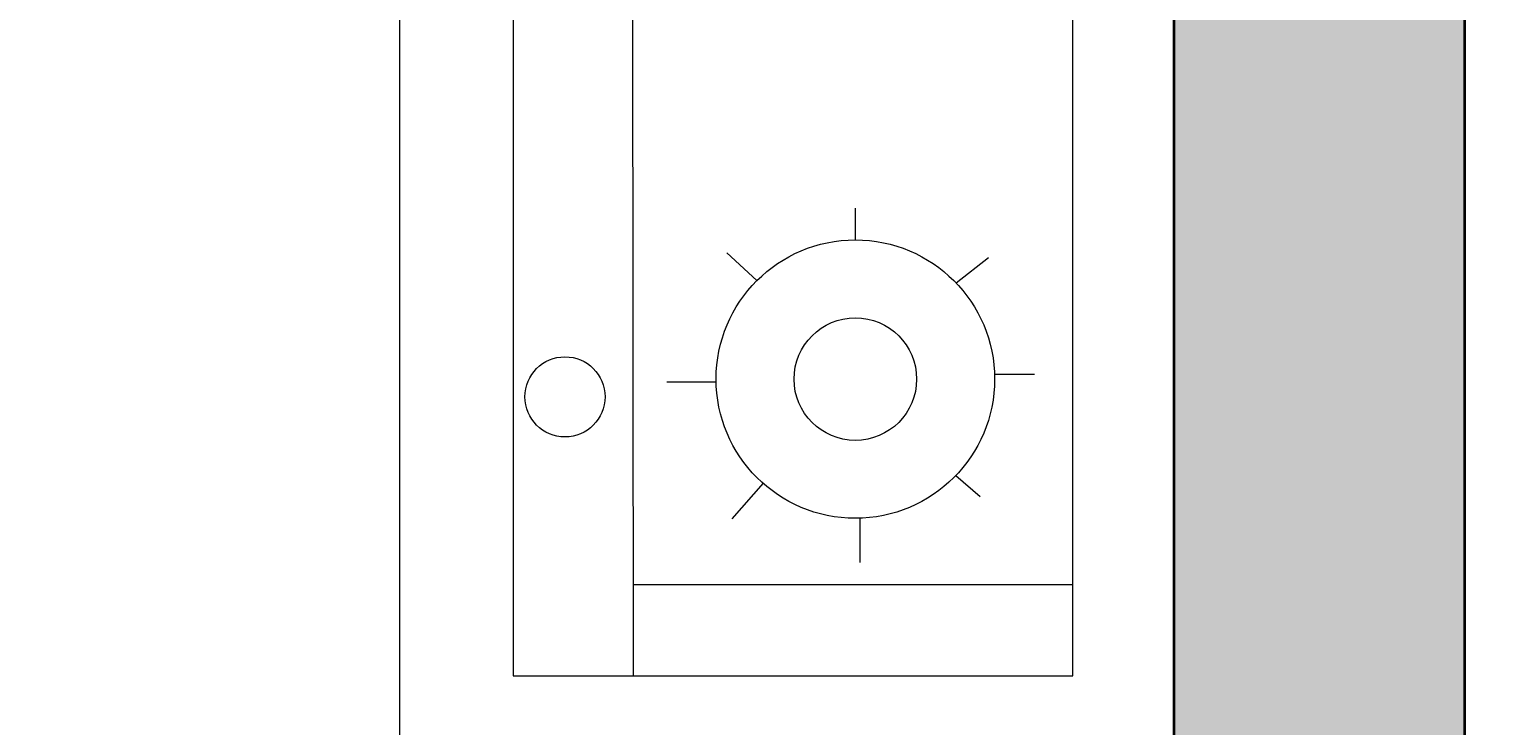
# Model space of a CAD drawing. Units: inches. Extents: x 1568 to 2529, y 2149 to 2897.
# Tile 5 of 16: x 1929 to 1974, y 2364 to 2386. Entities that reach past the tile are written whole.
import ezdxf

# ---------------------------------------------------------------- set-up
doc = ezdxf.new("R2010")
doc.units = ezdxf.units.IN
for name, color, linetype, lineweight in [('A-ANNO-DIMS', 2, 'Continuous', 18), ('A-EQPM', 8, 'Continuous', 18), ('A-FLOR-FIXT', 9, 'Continuous', 18), ('A-WALL-PATT', 172, 'Continuous', 13), ('wall', 7, 'Continuous', 35)]:
    doc.layers.add(name, color=color, linetype=linetype, lineweight=lineweight)
doc.styles.get("Standard").update_dxf_attribs({"font": 'arial.ttf'})
doc.dimstyles.get("Standard").update_dxf_attribs({"dimtxt": 0.18, "dimasz": 0.18, "dimexe": 0.18, "dimexo": 0.0625, "dimgap": 0.09, "dimtad": 0, "dimtih": 1, "dimtoh": 1, "dimdec": 4, "dimzin": 0, "dimdsep": 46, "dimtxsty": 'Standard', "dimcen": 0.09, "dimadec": 0, "dimazin": 0, "dimtfac": 1, "dimtdec": 4, "dimtofl": 0, "dimtmove": 0, "dimatfit": 3, "dimfxl": 1, "dimtolj": 1, "dimtzin": 0, "dimarcsym": 0})

# ---------------------------------------------------------------- blocks, each defined once
blk = doc.blocks.new('COOKTOP-BURNER')
for p, q in [((0.001, 4.315), (0.001, 5.296)), ((-3.048, 3.054), (-3.977, 3.91)), ((3.12, 2.981), (4.125, 3.765)), ((4.312, 0.148), (5.549, 0.148)), ((-4.314, -0.098), (-5.839, -0.098)), ((3.11, -2.99), (3.87, -3.639)), ((-2.86, -3.23), (-3.831, -4.332)), ((0.143, -4.312), (0.143, -5.681))]:
    blk.add_line(p, q)
for radius in [4.315, 1.899]:
    blk.add_circle((0, 0), radius)
blk = doc.blocks.new('*D28')
at = {"layer": 'A-ANNO-DIMS', "color": 0, "lineweight": -2, "transparency": 16777216}
for p, q in [((1973.643, 2801.532), (2009.61, 2801.532)), ((2009.43, 2801.352), (2009.43, 2501.714)), ((2009.43, 2201.712), (2009.43, 2501.35)), ((1973.613, 2201.532), (2009.61, 2201.532))]:
    blk.add_line(p, q, dxfattribs=at)
at = {"layer": 'A-ANNO-DIMS', "color": 0, "transparency": 16777216}
for points in [[(2009.4, 2801.352), (2009.46, 2801.352), (2009.43, 2801.532)], [(2009.4, 2201.712), (2009.46, 2201.712), (2009.43, 2201.532)]]:
    blk.add_solid(points, dxfattribs=at)
at = {"layer": 'Defpoints', "color": 0, "transparency": 16777216}
for p in [(1973.58, 2801.532), (2009.43, 2801.532), (1973.551, 2201.532)]:
    blk.add_point(p, dxfattribs=at)
at = {"layer": 'A-ANNO-DIMS', "color": 0, "transparency": 16777216, "insert": (2009.43, 2501.532), "char_height": 0.18, "attachment_point": 5}
blk.add_mtext('\\A1;600', dxfattribs=at)
blk = doc.blocks.new('*D32')
at = {"layer": 'A-ANNO-DIMS', "color": 0, "lineweight": -2, "transparency": 16777216}
for p, q in [((1964.551, 2792.469), (1964.551, 2165.502)), ((1904.551, 2753.401), (1904.551, 2165.502)), ((1904.731, 2165.682), (1934.332, 2165.682)), ((1964.371, 2165.682), (1934.77, 2165.682))]:
    blk.add_line(p, q, dxfattribs=at)
at = {"layer": 'A-ANNO-DIMS', "color": 0, "transparency": 16777216}
for points in [[(1904.731, 2165.712), (1904.731, 2165.652), (1904.551, 2165.682)], [(1964.371, 2165.712), (1964.371, 2165.652), (1964.551, 2165.682)]]:
    blk.add_solid(points, dxfattribs=at)
at = {"layer": 'Defpoints', "color": 0, "transparency": 16777216}
for p in [(1964.551, 2792.532), (1904.551, 2753.463), (1964.551, 2165.682)]:
    blk.add_point(p, dxfattribs=at)
at = {"layer": 'A-ANNO-DIMS', "color": 0, "transparency": 16777216, "insert": (1934.551, 2165.682), "char_height": 0.18, "attachment_point": 5}
blk.add_mtext('\\A1;60', dxfattribs=at)

msp = doc.modelspace()

# ---------------------------------------------------------------- hatches: boundary and pattern name
at = {"layer": 'A-WALL-PATT'}
h = msp.add_hatch(color=256, dxfattribs=at)
h.dxf.hatch_style = 1
h.paths.add_polyline_path([(1738.1593, 2801.532), (1634.4841, 2801.532), (1634.4841, 2792.532), (1738.1593, 2792.532)])
h.paths.add_polyline_path([(1812.4114, 2801.532), (1759.0925, 2801.532), (1759.0925, 2792.532), (1812.4114, 2792.532)])
h.paths.add_polyline_path([(1952.647, 2801.532), (1848.4114, 2801.532), (1848.4114, 2792.532), (1952.647, 2792.532)])
h.paths.add_polyline_path([(1973.5509, 2792.532), (1964.5509, 2792.532), (1964.5509, 2699.1671), (1973.5509, 2699.1671)])
h.paths.add_polyline_path([(1973.5509, 2663.1671), (1964.5509, 2663.1671), (1964.5509, 2630.5978), (1973.5509, 2630.5978)])
h.paths.add_polyline_path([(1973.5509, 2609.6646), (1964.5509, 2609.6646), (1964.5509, 2572.3679), (1973.5509, 2572.3679)])
h.paths.add_polyline_path([(1622.5509, 2753.3576), (1622.3864, 2753.3576), (1613.5509, 2753.3576), (1613.5509, 2705.9172), (1622.5509, 2705.9172)])
h.paths.add_polyline_path([(1622.5509, 2669.9172), (1613.5509, 2669.9172), (1613.5509, 2624.532), (1622.5509, 2624.532)])
h.paths.add_polyline_path([(1759.0509, 2757.9833), (1754.5509, 2757.9833), (1754.5509, 2744.532), (1622.5509, 2744.532), (1622.5509, 2740.032), (1754.5509, 2740.032), (1754.5509, 2730.8156), (1759.0509, 2730.8156), (1759.0509, 2740.032)])
h.paths.add_polyline_path([(1759.0509, 2690.8156), (1754.5509, 2690.8156), (1754.5509, 2624.532), (1759.0509, 2624.532)])
h.paths.add_polyline_path([(1738.1177, 2620.032), (1634.4841, 2620.032), (1634.4841, 2615.532), (1738.1177, 2615.532)])
h.paths.add_polyline_path([(1622.5509, 2615.532), (1613.5509, 2615.532), (1613.5509, 2564.2764), (1622.5509, 2564.2764)])
h.paths.add_polyline_path([(1759.0509, 2411.2271), (1754.5509, 2411.2271), (1754.5509, 2339.532), (1759.0509, 2339.532)])
h.paths.add_polyline_path([(1759.0509, 2464.032), (1734.3925, 2464.032), (1622.5509, 2464.032), (1622.5509, 2459.532), (1736.5509, 2459.532), (1754.5509, 2459.532), (1754.5509, 2451.2271), (1759.0509, 2451.2271)])
h.paths.add_polyline_path([(1844.5509, 2471.532), (1858.1805, 2471.532), (1858.1805, 2476.032), (1844.5509, 2476.032), (1844.5509, 2510.0763), (1840.0509, 2510.0763), (1840.0509, 2476.032), (1840.0509, 2339.532), (1844.5509, 2339.532)])
h.paths.add_polyline_path([(1844.5509, 2596.032), (1964.5509, 2596.032), (1964.5509, 2600.532), (1840.0509, 2600.532), (1840.0509, 2570.0763), (1844.5509, 2570.0763)])
h.paths.add_polyline_path([(1964.5509, 2476.032), (1894.1805, 2476.032), (1894.1805, 2471.532), (1964.5509, 2471.532)])
h.paths.add_polyline_path([(1622.5509, 2528.2764), (1613.5509, 2528.2764), (1613.5509, 2436.512), (1622.5509, 2436.512)])
h.paths.add_polyline_path([(1622.5509, 2400.512), (1613.5509, 2400.512), (1613.5509, 2339.532), (1622.5509, 2339.532)])
h.paths.add_polyline_path([(1738.9144, 2339.532), (1634.4841, 2339.532), (1634.4841, 2330.532), (1738.9144, 2330.532)])
h.paths.add_polyline_path([(1792.463, 2336.532, -0.0187698), (1792.5756, 2339.532), (1783.8928, 2339.532), (1783.8928, 2330.532), (1792.463, 2330.532)])
h.paths.add_polyline_path([(1952.6177, 2339.532), (1885.2912, 2339.532), (1885.2912, 2330.532), (1952.6177, 2330.532)])
h.paths.add_polyline_path([(1973.5509, 2422.371), (1964.5509, 2422.371), (1964.5509, 2395.032), (1964.5509, 2387.286), (1964.5509, 2339.532), (1973.5509, 2339.532)])
h.paths.add_polyline_path([(1973.5509, 2536.3679), (1964.5509, 2536.3679), (1964.5509, 2476.032), (1964.5509, 2458.371), (1973.5509, 2458.371)])

# ---------------------------------------------------------------- linework, layer by layer
at = {"layer": 'A-EQPM'}
for p, q in [((1947.7496, 2399.6535), (1947.7862, 2365.7088)), ((1947.7832, 2368.544), (1961.4053, 2368.544))]:
    msp.add_line(p, q, dxfattribs=at)
msp.add_lwpolyline([(1944.063, 2365.7088), (1961.4053, 2365.7088), (1961.4053, 2399.6535), (1944.063, 2399.6535)], close=True, dxfattribs=at)
msp.add_circle((1945.6729, 2374.3571), 1.2412, dxfattribs=at)
at = {"layer": 'A-FLOR-FIXT'}
msp.add_line((1940.5509, 2471.532), (1940.5509, 2339.532), dxfattribs=at)
at = {"layer": 'wall'}
msp.add_lwpolyline([(1613.5509, 2201.532), (1973.5509, 2201.532), (1973.5509, 2801.532), (1613.5509, 2801.532)], close=True, dxfattribs=at)
msp.add_lwpolyline([(1964.5509, 2339.532), (1964.5509, 2390.532)], dxfattribs=at)

# ---------------------------------------------------------------- block references
at = {"layer": 'A-EQPM'}
msp.add_blockref('COOKTOP-BURNER', (1954.6696, 2374.9077), dxfattribs=at)

# ---------------------------------------------------------------- dimensions: what is measured, and where the dimension line sits
at = {"layer": 'A-ANNO-DIMS'}
dim = msp.add_linear_dim(base=(2009.4302, 2801.532), p1=(1973.5509, 2201.532), p2=(1973.5802, 2801.532), angle=90, dimstyle='Standard', override={"dimdec": 0, "dimlfac": 1, "dimrnd": 0, "dimzin": 0, "dimdsep": 46, "dimlunit": 2}, dxfattribs=at)
dim.commit()
dim.dimension.update_dxf_attribs({"geometry": '*D28', "text_midpoint": (2009.4302, 2501.532)})
dim = msp.add_linear_dim(base=(1964.5509, 2165.682), p1=(1904.5509, 2753.4635), p2=(1964.5509, 2792.532), dimstyle='Standard', override={"dimdec": 0, "dimlfac": 1, "dimrnd": 0, "dimzin": 0, "dimdsep": 46, "dimlunit": 2}, dxfattribs=at)
dim.commit()
dim.dimension.update_dxf_attribs({"geometry": '*D32', "text_midpoint": (1934.5509, 2165.682)})

doc.saveas('drawing.dxf')
